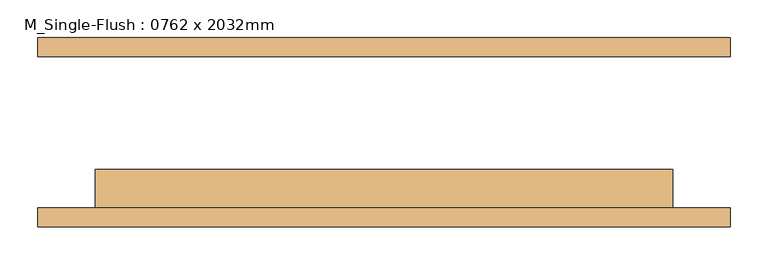
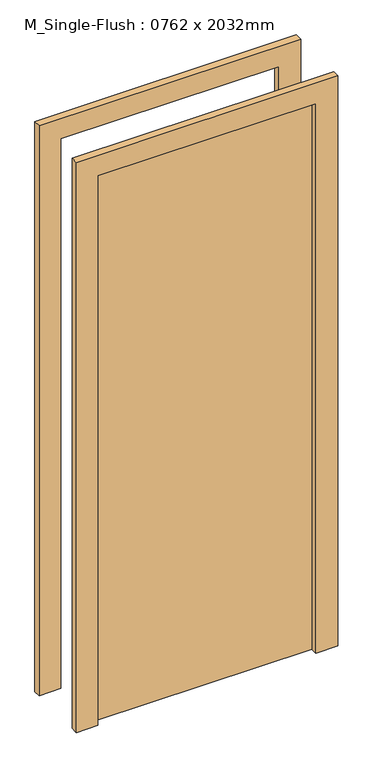
"""IFC4 building model written with IfcOpenShell, lengths in millimetres: door geometry, M_Single-Flush : 0762 x 2032mm."""

from ifc_helpers import new_model, si_unit, frame, origin, origin_with_axes, place, context, project, spatial, polyline, outline, extrude, source, transform, mapped, element, save


def m_single_flush_0762_x_2032mm_7341a4fb(model_context):
    return source(origin(), model_context, "Body", "SweptSolid", [
        extrude(outline(polyline([(2108.0, -457.0), (0.0, -457.0), (0.0, -381.0), (2032.0, -381.0), (2032.0, 381.0), (0.0, 381.0), (0.0, 457.0), (2108.0, 457.0), (2108.0, -457.0)])), frame((0.0, -125.0, 0.0), z_axis=(0.0, 1.0, 0.0), x_axis=(0.0, 0.0, 1.0)), (0.0, 0.0, 1.0), 25.0),
        extrude(outline(polyline([(2108.0, 457.0), (2108.0, -457.0), (0.0, -457.0), (0.0, -381.0), (2032.0, -381.0), (2032.0, 381.0), (0.0, 381.0), (0.0, 457.0), (2108.0, 457.0)])), frame((0.0, 100.0, 0.0), z_axis=(0.0, 1.0, 0.0), x_axis=(0.0, 0.0, 1.0)), (0.0, 0.0, 1.0), 25.0),
        extrude(outline(polyline([(381.0, -49.0), (381.0, -100.0), (-381.0, -100.0), (-381.0, -49.0), (381.0, -49.0)])), origin_with_axes(), (0.0, 0.0, 1.0), 2032.0),
    ])


if __name__ == "__main__":
    model = new_model("IFC4")
    model_context = context("Model", 3, world=origin())
    ifc_project = project(units=[si_unit("LENGTHUNIT", "METRE", prefix="MILLI")], contexts=[model_context])
    site = spatial("IfcSite", under=ifc_project)
    building = spatial("IfcBuilding", under=site)
    placement = place(None, origin())
    m_single_flush_0762_x_2032mm_shape = m_single_flush_0762_x_2032mm_7341a4fb(model_context)
    element("IfcDoor", 1, ObjectType="M_Single-Flush : 0762 x 2032mm", at=placement, inside=building, context=model_context, shape_type="MappedRepresentation", body=[
        mapped(m_single_flush_0762_x_2032mm_shape, transform((0.0, 0.0, 0.0), x_axis=(1.0, 0.0, 0.0), y_axis=(0.0, 1.0, 0.0), z_axis=(0.0, 0.0, 1.0))),
    ])
    save(model, "model.ifc")

# Revit data of these elements
# Type "M_Single-Flush : 0762 x 2032mm"
#   Type Mark = "19"
#   Thickness = 51 mm
#   Height = 2032 mm
#   Trim Projection Ext = 25 mm
#   Trim Projection Int = 25 mm
#   Trim Width = 76 mm
#   Width = 762 mm
#   Door Material = Door - Panel
#   Frame Material = Door - Frame
#   Function = (empty or 0)
#   Wall Closure = (empty or 0)
# Element 1 (IfcDoor, "M_Single-Flush : 0762 x 2032mm")
#   Materials on its faces: "Door - Frame", "Door - Panel"
# Materials
#   "Door - Panel": class "Wood", colour RGB 114 82 51, transparency 0
#   "Door - Frame": colour RGB 153 76 43, transparency 0
